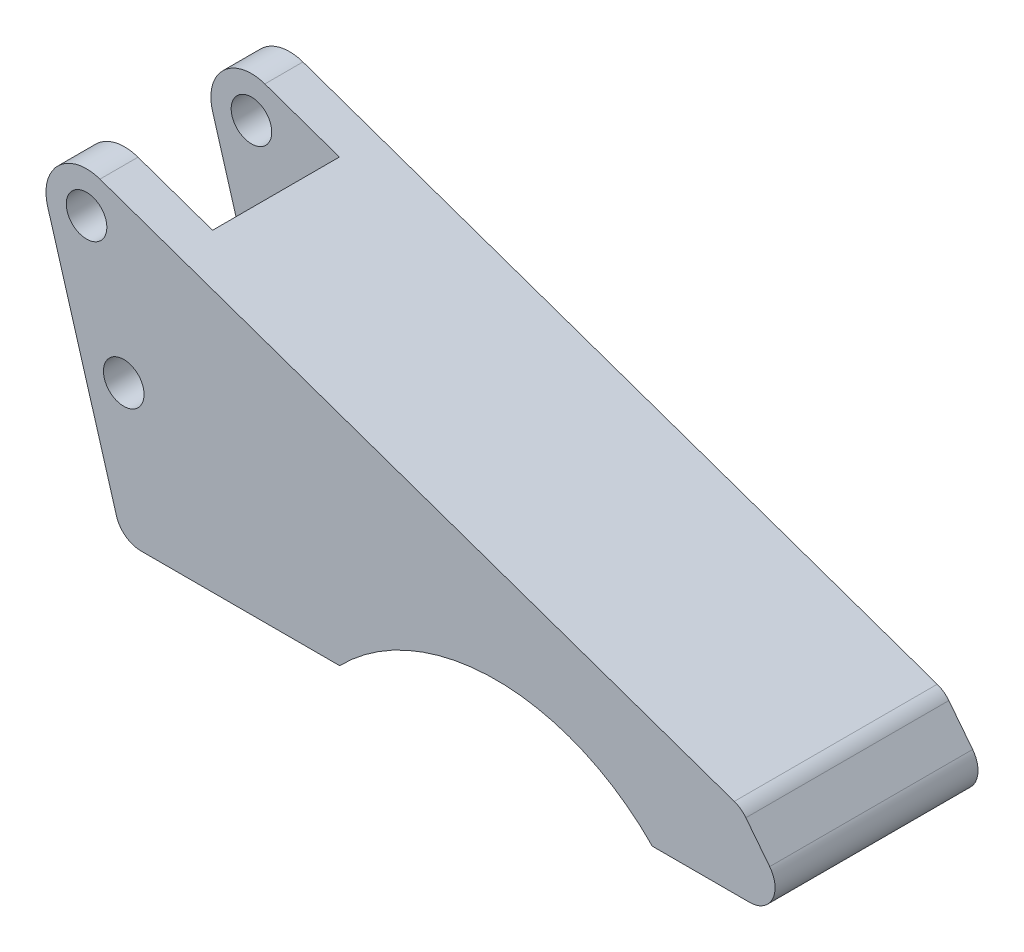
ISO-10303-21;
HEADER;
FILE_DESCRIPTION(('STEP AP214'),'2;1');
FILE_NAME('part.step','',(''),(''),'','','');
FILE_SCHEMA(('AUTOMOTIVE_DESIGN { 1 0 10303 214 1 1 1 1 }'));
ENDSEC;
DATA;
#1=APPLICATION_CONTEXT('core data for automotive mechanical design processes');
#2=APPLICATION_PROTOCOL_DEFINITION('international standard','automotive_design',2000,#1);
#3=PRODUCT_CONTEXT('',#1,'mechanical');
#4=PRODUCT('Part','Part','',(#3));
#5=PRODUCT_RELATED_PRODUCT_CATEGORY('part','',(#4));
#6=PRODUCT_DEFINITION_FORMATION('','',#4);
#7=PRODUCT_DEFINITION_CONTEXT('part definition',#1,'design');
#8=PRODUCT_DEFINITION('design','',#6,#7);
#9=PRODUCT_DEFINITION_SHAPE('','',#8);
#10=(LENGTH_UNIT() NAMED_UNIT(*) SI_UNIT(.MILLI.,.METRE.));
#11=(NAMED_UNIT(*) PLANE_ANGLE_UNIT() SI_UNIT($,.RADIAN.));
#12=(NAMED_UNIT(*) SI_UNIT($,.STERADIAN.) SOLID_ANGLE_UNIT());
#13=UNCERTAINTY_MEASURE_WITH_UNIT(LENGTH_MEASURE(1.E-05),#10,'distance_accuracy_value','');
#14=(GEOMETRIC_REPRESENTATION_CONTEXT(3) GLOBAL_UNCERTAINTY_ASSIGNED_CONTEXT((#13)) GLOBAL_UNIT_ASSIGNED_CONTEXT((#10,
#11,#12)) REPRESENTATION_CONTEXT('',''));
#15=CARTESIAN_POINT('',(0.,0.,0.));
#16=DIRECTION('',(0.,0.,1.));
#17=DIRECTION('',(1.,0.,0.));
#18=AXIS2_PLACEMENT_3D('',#15,#16,#17);
#19=CARTESIAN_POINT('',(-49.8841563985013,51.87,20.));
#20=DIRECTION('',(0.,0.,-1.));
#21=DIRECTION('',(-1.,0.,0.));
#22=AXIS2_PLACEMENT_3D('',#19,#20,#21);
#23=CYLINDRICAL_SURFACE('',#22,7.99999999999999);
#24=CARTESIAN_POINT('',(-49.8841563985013,51.87,12.5));
#25=DIRECTION('',(0.,0.,1.));
#26=DIRECTION('',(1.,0.,0.));
#27=AXIS2_PLACEMENT_3D('',#24,#25,#26);
#28=CIRCLE('',#27,7.99999999999999);
#29=CARTESIAN_POINT('',(-47.2441563985013,59.4218474560865,12.5));
#30=VERTEX_POINT('',#29);
#31=CARTESIAN_POINT('',(-57.5576448104909,49.6077940873871,12.5));
#32=VERTEX_POINT('',#31);
#33=EDGE_CURVE('E230',#30,#32,#28,.T.);
#34=ORIENTED_EDGE('',*,*,#33,.T.);
#35=DIRECTION('',(0.,0.,-1.));
#36=VECTOR('',#35,1.);
#37=CARTESIAN_POINT('',(-57.5576448104909,49.6077940873871,20.));
#38=LINE('',#37,#36);
#39=CARTESIAN_POINT('',(-57.5576448104909,49.6077940873871,20.));
#40=VERTEX_POINT('',#39);
#41=EDGE_CURVE('E192',#40,#32,#38,.T.);
#42=ORIENTED_EDGE('',*,*,#41,.F.);
#43=CARTESIAN_POINT('',(-49.8841563985013,51.87,20.));
#44=DIRECTION('',(0.,0.,1.));
#45=DIRECTION('',(1.,0.,0.));
#46=AXIS2_PLACEMENT_3D('',#43,#44,#45);
#47=CIRCLE('',#46,7.99999999999999);
#48=CARTESIAN_POINT('',(-47.2441563985013,59.4218474560865,20.));
#49=VERTEX_POINT('',#48);
#50=EDGE_CURVE('E143',#49,#40,#47,.T.);
#51=ORIENTED_EDGE('',*,*,#50,.F.);
#52=DIRECTION('',(0.,0.,-1.));
#53=VECTOR('',#52,1.);
#54=CARTESIAN_POINT('',(-47.2441563985013,59.4218474560865,20.));
#55=LINE('',#54,#53);
#56=EDGE_CURVE('E196',#49,#30,#55,.T.);
#57=ORIENTED_EDGE('',*,*,#56,.T.);
#58=EDGE_LOOP('',(#34,#42,#51,#57));
#59=FACE_BOUND('',#58,.T.);
#60=ADVANCED_FACE('F41',(#59),#23,.T.);
#61=CARTESIAN_POINT('',(-43.9900866559948,3.5861213046169,20.));
#62=DIRECTION('',(0.959186051498703,0.282775739076619,0.));
#63=DIRECTION('',(-0.282775739076619,0.959186051498703,0.));
#64=AXIS2_PLACEMENT_3D('',#61,#62,#63);
#65=PLANE('',#64);
#66=DIRECTION('',(0.,0.,-1.));
#67=VECTOR('',#66,1.);
#68=CARTESIAN_POINT('',(-43.9900866559948,3.5861213046169,20.));
#69=LINE('',#68,#67);
#70=CARTESIAN_POINT('',(-43.9900866559948,3.5861213046169,-12.5));
#71=VERTEX_POINT('',#70);
#72=CARTESIAN_POINT('',(-43.9900866559948,3.5861213046169,-20.));
#73=VERTEX_POINT('',#72);
#74=EDGE_CURVE('E156',#71,#73,#69,.T.);
#75=ORIENTED_EDGE('',*,*,#74,.F.);
#76=DIRECTION('',(-0.282775739076619,0.959186051498703,0.));
#77=VECTOR('',#76,1.);
#78=CARTESIAN_POINT('',(-43.9900866559948,3.5861213046169,-12.5));
#79=LINE('',#78,#77);
#80=CARTESIAN_POINT('',(-57.5576448104909,49.6077940873871,-12.5));
#81=VERTEX_POINT('',#80);
#82=EDGE_CURVE('E245',#71,#81,#79,.T.);
#83=ORIENTED_EDGE('',*,*,#82,.T.);
#84=CARTESIAN_POINT('',(-57.5576448104909,49.6077940873871,-20.));
#85=VERTEX_POINT('',#84);
#86=EDGE_CURVE('E154',#81,#85,#38,.T.);
#87=ORIENTED_EDGE('',*,*,#86,.T.);
#88=DIRECTION('',(0.282775739076619,-0.959186051498703,0.));
#89=VECTOR('',#88,1.);
#90=CARTESIAN_POINT('',(-43.9900866559948,3.5861213046169,-20.));
#91=LINE('',#90,#89);
#92=EDGE_CURVE('E184',#85,#73,#91,.T.);
#93=ORIENTED_EDGE('',*,*,#92,.T.);
#94=EDGE_LOOP('',(#75,#83,#87,#93));
#95=FACE_BOUND('',#94,.T.);
#96=ADVANCED_FACE('F321',(#95),#65,.F.);
#97=CARTESIAN_POINT('',(-39.1941563985013,5.,20.));
#98=DIRECTION('',(0.,0.,-1.));
#99=DIRECTION('',(-1.,0.,0.));
#100=AXIS2_PLACEMENT_3D('',#97,#98,#99);
#101=CYLINDRICAL_SURFACE('',#100,5.);
#102=DIRECTION('',(0.,0.,-1.));
#103=VECTOR('',#102,1.);
#104=CARTESIAN_POINT('',(-39.1941563985013,0.,20.));
#105=LINE('',#104,#103);
#106=CARTESIAN_POINT('',(-39.1941563985013,0.,-12.5));
#107=VERTEX_POINT('',#106);
#108=CARTESIAN_POINT('',(-39.1941563985013,0.,-20.));
#109=VERTEX_POINT('',#108);
#110=EDGE_CURVE('E195',#107,#109,#105,.T.);
#111=ORIENTED_EDGE('',*,*,#110,.F.);
#112=CARTESIAN_POINT('',(-39.1941563985013,5.,-12.5));
#113=DIRECTION('',(0.,0.,-1.));
#114=DIRECTION('',(-1.,0.,0.));
#115=AXIS2_PLACEMENT_3D('',#112,#113,#114);
#116=CIRCLE('',#115,5.);
#117=EDGE_CURVE('E238',#107,#71,#116,.T.);
#118=ORIENTED_EDGE('',*,*,#117,.T.);
#119=ORIENTED_EDGE('',*,*,#74,.T.);
#120=CARTESIAN_POINT('',(-39.1941563985013,5.,-20.));
#121=DIRECTION('',(0.,0.,1.));
#122=DIRECTION('',(-1.,0.,0.));
#123=AXIS2_PLACEMENT_3D('',#120,#121,#122);
#124=CIRCLE('',#123,5.);
#125=EDGE_CURVE('E186',#73,#109,#124,.T.);
#126=ORIENTED_EDGE('',*,*,#125,.T.);
#127=EDGE_LOOP('',(#111,#118,#119,#126));
#128=FACE_BOUND('',#127,.T.);
#129=ADVANCED_FACE('F322',(#128),#101,.T.);
#130=CARTESIAN_POINT('',(-49.8841563985013,51.87,20.));
#131=DIRECTION('',(0.,0.,-1.));
#132=DIRECTION('',(-1.,0.,0.));
#133=AXIS2_PLACEMENT_3D('',#130,#131,#132);
#134=CYLINDRICAL_SURFACE('',#133,3.99999999999999);
#135=CARTESIAN_POINT('',(-49.8841563985013,51.87,-12.5));
#136=DIRECTION('',(0.,0.,-1.));
#137=DIRECTION('',(-1.,0.,0.));
#138=AXIS2_PLACEMENT_3D('',#135,#136,#137);
#139=CIRCLE('',#138,3.99999999999999);
#140=CARTESIAN_POINT('',(-53.8841563985013,51.87,-12.5));
#141=VERTEX_POINT('',#140);
#142=EDGE_CURVE('E219',#141,#141,#139,.T.);
#143=ORIENTED_EDGE('',*,*,#142,.F.);
#144=EDGE_LOOP('',(#143));
#145=FACE_BOUND('',#144,.T.);
#146=CARTESIAN_POINT('',(-49.8841563985013,51.87,-20.));
#147=DIRECTION('',(0.,0.,1.));
#148=DIRECTION('',(1.,0.,0.));
#149=AXIS2_PLACEMENT_3D('',#146,#147,#148);
#150=CIRCLE('',#149,3.99999999999999);
#151=CARTESIAN_POINT('',(-45.8841563985013,51.87,-20.));
#152=VERTEX_POINT('',#151);
#153=EDGE_CURVE('E256',#152,#152,#150,.T.);
#154=ORIENTED_EDGE('',*,*,#153,.F.);
#155=EDGE_LOOP('',(#154));
#156=FACE_BOUND('',#155,.T.);
#157=ADVANCED_FACE('F388',(#145,#156),#134,.F.);
#158=CARTESIAN_POINT('',(-42.5541563985013,27.,20.));
#159=DIRECTION('',(0.,0.,-1.));
#160=DIRECTION('',(-1.,0.,0.));
#161=AXIS2_PLACEMENT_3D('',#158,#159,#160);
#162=CYLINDRICAL_SURFACE('',#161,4.);
#163=CARTESIAN_POINT('',(-42.5541563985013,27.,-12.5));
#164=DIRECTION('',(0.,0.,-1.));
#165=DIRECTION('',(-1.,0.,0.));
#166=AXIS2_PLACEMENT_3D('',#163,#164,#165);
#167=CIRCLE('',#166,4.);
#168=CARTESIAN_POINT('',(-46.5541563985013,27.,-12.5));
#169=VERTEX_POINT('',#168);
#170=EDGE_CURVE('E217',#169,#169,#167,.T.);
#171=ORIENTED_EDGE('',*,*,#170,.F.);
#172=EDGE_LOOP('',(#171));
#173=FACE_BOUND('',#172,.T.);
#174=CARTESIAN_POINT('',(-42.5541563985013,27.,-20.));
#175=DIRECTION('',(0.,0.,1.));
#176=DIRECTION('',(1.,0.,0.));
#177=AXIS2_PLACEMENT_3D('',#174,#175,#176);
#178=CIRCLE('',#177,4.);
#179=CARTESIAN_POINT('',(-38.5541563985013,27.,-20.));
#180=VERTEX_POINT('',#179);
#181=EDGE_CURVE('E255',#180,#180,#178,.T.);
#182=ORIENTED_EDGE('',*,*,#181,.F.);
#183=EDGE_LOOP('',(#182));
#184=FACE_BOUND('',#183,.T.);
#185=ADVANCED_FACE('F384',(#173,#184),#162,.F.);
#186=CARTESIAN_POINT('',(30.8058436014987,-30.,20.));
#187=DIRECTION('',(0.,0.,-1.));
#188=DIRECTION('',(-1.,0.,0.));
#189=AXIS2_PLACEMENT_3D('',#186,#187,#188);
#190=PLANE('',#189);
#191=CARTESIAN_POINT('',(30.8058436014987,-30.,20.));
#192=DIRECTION('',(0.,0.,-1.));
#193=DIRECTION('',(-1.,0.,0.));
#194=AXIS2_PLACEMENT_3D('',#191,#192,#193);
#195=CIRCLE('',#194,43.);
#196=CARTESIAN_POINT('',(0.,0.,20.));
#197=VERTEX_POINT('',#196);
#198=CARTESIAN_POINT('',(61.6116872029974,0.,20.));
#199=VERTEX_POINT('',#198);
#200=EDGE_CURVE('E194',#197,#199,#195,.T.);
#201=ORIENTED_EDGE('',*,*,#200,.T.);
#202=DIRECTION('',(1.,0.,0.));
#203=VECTOR('',#202,1.);
#204=CARTESIAN_POINT('',(61.6116872029974,0.,20.));
#205=LINE('',#204,#203);
#206=CARTESIAN_POINT('',(80.8058436014987,0.,20.));
#207=VERTEX_POINT('',#206);
#208=EDGE_CURVE('E115',#199,#207,#205,.T.);
#209=ORIENTED_EDGE('',*,*,#208,.T.);
#210=CARTESIAN_POINT('',(80.8058436014987,5.,20.));
#211=DIRECTION('',(0.,0.,1.));
#212=DIRECTION('',(1.,0.,0.));
#213=AXIS2_PLACEMENT_3D('',#210,#211,#212);
#214=CIRCLE('',#213,5.);
#215=CARTESIAN_POINT('',(84.7456523822993,8.07862092027041,20.));
#216=VERTEX_POINT('',#215);
#217=EDGE_CURVE('E270',#207,#216,#214,.T.);
#218=ORIENTED_EDGE('',*,*,#217,.T.);
#219=DIRECTION('',(-0.615724184054082,0.787961756160116,0.));
#220=VECTOR('',#219,1.);
#221=CARTESIAN_POINT('',(80.0571696286086,14.0786209202704,20.));
#222=LINE('',#221,#220);
#223=CARTESIAN_POINT('',(80.0571696286086,14.0786209202704,20.));
#224=VERTEX_POINT('',#223);
#225=EDGE_CURVE('E267',#216,#224,#222,.T.);
#226=ORIENTED_EDGE('',*,*,#225,.T.);
#227=CARTESIAN_POINT('',(76.1173608478081,11.,20.));
#228=DIRECTION('',(0.,0.,1.));
#229=DIRECTION('',(-1.,0.,0.));
#230=AXIS2_PLACEMENT_3D('',#227,#228,#229);
#231=CIRCLE('',#230,5.);
#232=CARTESIAN_POINT('',(77.767360847808,15.7199046600541,20.));
#233=VERTEX_POINT('',#232);
#234=EDGE_CURVE('E271',#224,#233,#231,.T.);
#235=ORIENTED_EDGE('',*,*,#234,.T.);
#236=DIRECTION('',(-0.943980932010812,0.329999999999998,0.));
#237=VECTOR('',#236,1.);
#238=CARTESIAN_POINT('',(-47.2441563985013,59.4218474560865,20.));
#239=LINE('',#238,#237);
#240=EDGE_CURVE('E272',#233,#49,#239,.T.);
#241=ORIENTED_EDGE('',*,*,#240,.T.);
#242=ORIENTED_EDGE('',*,*,#50,.T.);
#243=DIRECTION('',(0.282775739076619,-0.959186051498703,0.));
#244=VECTOR('',#243,1.);
#245=CARTESIAN_POINT('',(-43.9900866559948,3.5861213046169,20.));
#246=LINE('',#245,#244);
#247=CARTESIAN_POINT('',(-43.9900866559948,3.5861213046169,20.));
#248=VERTEX_POINT('',#247);
#249=EDGE_CURVE('E135',#40,#248,#246,.T.);
#250=ORIENTED_EDGE('',*,*,#249,.T.);
#251=CARTESIAN_POINT('',(-39.1941563985013,5.,20.));
#252=DIRECTION('',(0.,0.,1.));
#253=DIRECTION('',(-1.,0.,0.));
#254=AXIS2_PLACEMENT_3D('',#251,#252,#253);
#255=CIRCLE('',#254,5.);
#256=CARTESIAN_POINT('',(-39.1941563985013,0.,20.));
#257=VERTEX_POINT('',#256);
#258=EDGE_CURVE('E140',#248,#257,#255,.T.);
#259=ORIENTED_EDGE('',*,*,#258,.T.);
#260=DIRECTION('',(1.,0.,0.));
#261=VECTOR('',#260,1.);
#262=CARTESIAN_POINT('',(-39.1941563985013,0.,20.));
#263=LINE('',#262,#261);
#264=EDGE_CURVE('E62',#257,#197,#263,.T.);
#265=ORIENTED_EDGE('',*,*,#264,.T.);
#266=EDGE_LOOP('',(#201,#209,#218,#226,#235,#241,#242,#250,#259,#265));
#267=FACE_BOUND('',#266,.T.);
#268=CARTESIAN_POINT('',(-49.8841563985013,51.87,20.));
#269=DIRECTION('',(0.,0.,1.));
#270=DIRECTION('',(1.,0.,0.));
#271=AXIS2_PLACEMENT_3D('',#268,#269,#270);
#272=CIRCLE('',#271,3.99999999999999);
#273=CARTESIAN_POINT('',(-45.8841563985013,51.87,20.));
#274=VERTEX_POINT('',#273);
#275=EDGE_CURVE('E168',#274,#274,#272,.T.);
#276=ORIENTED_EDGE('',*,*,#275,.F.);
#277=EDGE_LOOP('',(#276));
#278=FACE_BOUND('',#277,.T.);
#279=CARTESIAN_POINT('',(-42.5541563985013,27.,20.));
#280=DIRECTION('',(0.,0.,1.));
#281=DIRECTION('',(1.,0.,0.));
#282=AXIS2_PLACEMENT_3D('',#279,#280,#281);
#283=CIRCLE('',#282,4.);
#284=CARTESIAN_POINT('',(-38.5541563985013,27.,20.));
#285=VERTEX_POINT('',#284);
#286=EDGE_CURVE('E254',#285,#285,#283,.T.);
#287=ORIENTED_EDGE('',*,*,#286,.F.);
#288=EDGE_LOOP('',(#287));
#289=FACE_BOUND('',#288,.T.);
#290=ADVANCED_FACE('F132',(#267,#278,#289),#190,.F.);
#291=CARTESIAN_POINT('',(30.8058436014987,-30.,-20.));
#292=DIRECTION('',(0.,0.,-1.));
#293=DIRECTION('',(-1.,0.,0.));
#294=AXIS2_PLACEMENT_3D('',#291,#292,#293);
#295=PLANE('',#294);
#296=ORIENTED_EDGE('',*,*,#153,.T.);
#297=EDGE_LOOP('',(#296));
#298=FACE_BOUND('',#297,.T.);
#299=CARTESIAN_POINT('',(30.8058436014987,-30.,-20.));
#300=DIRECTION('',(0.,0.,-1.));
#301=DIRECTION('',(-1.,0.,0.));
#302=AXIS2_PLACEMENT_3D('',#299,#300,#301);
#303=CIRCLE('',#302,43.);
#304=CARTESIAN_POINT('',(0.,0.,-20.));
#305=VERTEX_POINT('',#304);
#306=CARTESIAN_POINT('',(61.6116872029974,0.,-20.));
#307=VERTEX_POINT('',#306);
#308=EDGE_CURVE('E167',#305,#307,#303,.T.);
#309=ORIENTED_EDGE('',*,*,#308,.F.);
#310=DIRECTION('',(1.,0.,0.));
#311=VECTOR('',#310,1.);
#312=CARTESIAN_POINT('',(-39.1941563985013,0.,-20.));
#313=LINE('',#312,#311);
#314=EDGE_CURVE('E103',#109,#305,#313,.T.);
#315=ORIENTED_EDGE('',*,*,#314,.F.);
#316=ORIENTED_EDGE('',*,*,#125,.F.);
#317=ORIENTED_EDGE('',*,*,#92,.F.);
#318=CARTESIAN_POINT('',(-49.8841563985013,51.87,-20.));
#319=DIRECTION('',(0.,0.,1.));
#320=DIRECTION('',(1.,0.,0.));
#321=AXIS2_PLACEMENT_3D('',#318,#319,#320);
#322=CIRCLE('',#321,7.99999999999999);
#323=CARTESIAN_POINT('',(-47.2441563985013,59.4218474560865,-20.));
#324=VERTEX_POINT('',#323);
#325=EDGE_CURVE('E182',#324,#85,#322,.T.);
#326=ORIENTED_EDGE('',*,*,#325,.F.);
#327=DIRECTION('',(-0.943980932010812,0.329999999999998,0.));
#328=VECTOR('',#327,1.);
#329=CARTESIAN_POINT('',(-47.2441563985013,59.4218474560865,-20.));
#330=LINE('',#329,#328);
#331=CARTESIAN_POINT('',(77.767360847808,15.7199046600541,-20.));
#332=VERTEX_POINT('',#331);
#333=EDGE_CURVE('E180',#332,#324,#330,.T.);
#334=ORIENTED_EDGE('',*,*,#333,.F.);
#335=CARTESIAN_POINT('',(76.1173608478081,11.,-20.));
#336=DIRECTION('',(0.,0.,1.));
#337=DIRECTION('',(-1.,0.,0.));
#338=AXIS2_PLACEMENT_3D('',#335,#336,#337);
#339=CIRCLE('',#338,5.);
#340=CARTESIAN_POINT('',(80.0571696286086,14.0786209202704,-20.));
#341=VERTEX_POINT('',#340);
#342=EDGE_CURVE('E179',#341,#332,#339,.T.);
#343=ORIENTED_EDGE('',*,*,#342,.F.);
#344=DIRECTION('',(-0.615724184054082,0.787961756160116,0.));
#345=VECTOR('',#344,1.);
#346=CARTESIAN_POINT('',(80.0571696286086,14.0786209202704,-20.));
#347=LINE('',#346,#345);
#348=CARTESIAN_POINT('',(84.7456523822993,8.07862092027041,-20.));
#349=VERTEX_POINT('',#348);
#350=EDGE_CURVE('E173',#349,#341,#347,.T.);
#351=ORIENTED_EDGE('',*,*,#350,.F.);
#352=CARTESIAN_POINT('',(80.8058436014987,5.,-20.));
#353=DIRECTION('',(0.,0.,1.));
#354=DIRECTION('',(1.,0.,0.));
#355=AXIS2_PLACEMENT_3D('',#352,#353,#354);
#356=CIRCLE('',#355,5.);
#357=CARTESIAN_POINT('',(80.8058436014987,0.,-20.));
#358=VERTEX_POINT('',#357);
#359=EDGE_CURVE('E171',#358,#349,#356,.T.);
#360=ORIENTED_EDGE('',*,*,#359,.F.);
#361=DIRECTION('',(1.,0.,0.));
#362=VECTOR('',#361,1.);
#363=CARTESIAN_POINT('',(61.6116872029974,0.,-20.));
#364=LINE('',#363,#362);
#365=EDGE_CURVE('E166',#307,#358,#364,.T.);
#366=ORIENTED_EDGE('',*,*,#365,.F.);
#367=EDGE_LOOP('',(#309,#315,#316,#317,#326,#334,#343,#351,#360,#366));
#368=FACE_BOUND('',#367,.T.);
#369=ORIENTED_EDGE('',*,*,#181,.T.);
#370=EDGE_LOOP('',(#369));
#371=FACE_BOUND('',#370,.T.);
#372=ADVANCED_FACE('F316',(#298,#368,#371),#295,.T.);
#373=CARTESIAN_POINT('',(30.8058436014987,-30.,20.));
#374=DIRECTION('',(0.,0.,-1.));
#375=DIRECTION('',(-1.,0.,0.));
#376=AXIS2_PLACEMENT_3D('',#373,#374,#375);
#377=CYLINDRICAL_SURFACE('',#376,43.);
#378=ORIENTED_EDGE('',*,*,#308,.T.);
#379=DIRECTION('',(0.,0.,-1.));
#380=VECTOR('',#379,1.);
#381=CARTESIAN_POINT('',(61.6116872029974,0.,20.));
#382=LINE('',#381,#380);
#383=EDGE_CURVE('E47',#199,#307,#382,.T.);
#384=ORIENTED_EDGE('',*,*,#383,.F.);
#385=ORIENTED_EDGE('',*,*,#200,.F.);
#386=DIRECTION('',(0.,0.,-1.));
#387=VECTOR('',#386,1.);
#388=CARTESIAN_POINT('',(0.,0.,20.));
#389=LINE('',#388,#387);
#390=EDGE_CURVE('E165',#197,#305,#389,.T.);
#391=ORIENTED_EDGE('',*,*,#390,.T.);
#392=EDGE_LOOP('',(#378,#384,#385,#391));
#393=FACE_BOUND('',#392,.T.);
#394=ADVANCED_FACE('F43',(#393),#377,.F.);
#395=CARTESIAN_POINT('',(61.6116872029974,0.,20.));
#396=DIRECTION('',(0.,1.,0.));
#397=DIRECTION('',(0.,0.,1.));
#398=AXIS2_PLACEMENT_3D('',#395,#396,#397);
#399=PLANE('',#398);
#400=ORIENTED_EDGE('',*,*,#365,.T.);
#401=DIRECTION('',(0.,0.,-1.));
#402=VECTOR('',#401,1.);
#403=CARTESIAN_POINT('',(80.8058436014987,0.,20.));
#404=LINE('',#403,#402);
#405=EDGE_CURVE('E209',#207,#358,#404,.T.);
#406=ORIENTED_EDGE('',*,*,#405,.F.);
#407=ORIENTED_EDGE('',*,*,#208,.F.);
#408=ORIENTED_EDGE('',*,*,#383,.T.);
#409=EDGE_LOOP('',(#400,#406,#407,#408));
#410=FACE_BOUND('',#409,.T.);
#411=ADVANCED_FACE('F345',(#410),#399,.F.);
#412=CARTESIAN_POINT('',(80.8058436014987,5.,20.));
#413=DIRECTION('',(0.,0.,-1.));
#414=DIRECTION('',(-1.,0.,0.));
#415=AXIS2_PLACEMENT_3D('',#412,#413,#414);
#416=CYLINDRICAL_SURFACE('',#415,5.);
#417=ORIENTED_EDGE('',*,*,#359,.T.);
#418=DIRECTION('',(0.,0.,-1.));
#419=VECTOR('',#418,1.);
#420=CARTESIAN_POINT('',(84.7456523822993,8.07862092027041,20.));
#421=LINE('',#420,#419);
#422=EDGE_CURVE('E210',#216,#349,#421,.T.);
#423=ORIENTED_EDGE('',*,*,#422,.F.);
#424=ORIENTED_EDGE('',*,*,#217,.F.);
#425=ORIENTED_EDGE('',*,*,#405,.T.);
#426=EDGE_LOOP('',(#417,#423,#424,#425));
#427=FACE_BOUND('',#426,.T.);
#428=ADVANCED_FACE('F347',(#427),#416,.T.);
#429=CARTESIAN_POINT('',(80.0571696286086,14.0786209202704,20.));
#430=DIRECTION('',(-0.787961756160116,-0.615724184054082,0.));
#431=DIRECTION('',(0.615724184054082,-0.787961756160116,0.));
#432=AXIS2_PLACEMENT_3D('',#429,#430,#431);
#433=PLANE('',#432);
#434=ORIENTED_EDGE('',*,*,#350,.T.);
#435=DIRECTION('',(0.,0.,-1.));
#436=VECTOR('',#435,1.);
#437=CARTESIAN_POINT('',(80.0571696286086,14.0786209202704,20.));
#438=LINE('',#437,#436);
#439=EDGE_CURVE('E204',#224,#341,#438,.T.);
#440=ORIENTED_EDGE('',*,*,#439,.F.);
#441=ORIENTED_EDGE('',*,*,#225,.F.);
#442=ORIENTED_EDGE('',*,*,#422,.T.);
#443=EDGE_LOOP('',(#434,#440,#441,#442));
#444=FACE_BOUND('',#443,.T.);
#445=ADVANCED_FACE('F354',(#444),#433,.F.);
#446=CARTESIAN_POINT('',(76.1173608478081,11.,20.));
#447=DIRECTION('',(0.,0.,-1.));
#448=DIRECTION('',(-1.,0.,0.));
#449=AXIS2_PLACEMENT_3D('',#446,#447,#448);
#450=CYLINDRICAL_SURFACE('',#449,5.);
#451=ORIENTED_EDGE('',*,*,#342,.T.);
#452=DIRECTION('',(0.,0.,-1.));
#453=VECTOR('',#452,1.);
#454=CARTESIAN_POINT('',(77.767360847808,15.7199046600541,20.));
#455=LINE('',#454,#453);
#456=EDGE_CURVE('E203',#233,#332,#455,.T.);
#457=ORIENTED_EDGE('',*,*,#456,.F.);
#458=ORIENTED_EDGE('',*,*,#234,.F.);
#459=ORIENTED_EDGE('',*,*,#439,.T.);
#460=EDGE_LOOP('',(#451,#457,#458,#459));
#461=FACE_BOUND('',#460,.T.);
#462=ADVANCED_FACE('F355',(#461),#450,.T.);
#463=CARTESIAN_POINT('',(-47.2441563985013,59.4218474560865,20.));
#464=DIRECTION('',(-0.329999999999998,-0.943980932010812,0.));
#465=DIRECTION('',(0.943980932010812,-0.329999999999998,0.));
#466=AXIS2_PLACEMENT_3D('',#463,#464,#465);
#467=PLANE('',#466);
#468=CARTESIAN_POINT('',(-47.2441563985013,59.4218474560865,-12.5));
#469=VERTEX_POINT('',#468);
#470=EDGE_CURVE('E197',#469,#324,#55,.T.);
#471=ORIENTED_EDGE('',*,*,#470,.F.);
#472=DIRECTION('',(0.943980932010812,-0.329999999999998,0.));
#473=VECTOR('',#472,1.);
#474=CARTESIAN_POINT('',(-47.2441563985013,59.4218474560865,-12.5));
#475=LINE('',#474,#473);
#476=CARTESIAN_POINT('',(-32.5576448104909,54.287687792798,-12.5));
#477=VERTEX_POINT('',#476);
#478=EDGE_CURVE('E248',#469,#477,#475,.T.);
#479=ORIENTED_EDGE('',*,*,#478,.T.);
#480=DIRECTION('',(0.,0.,1.));
#481=VECTOR('',#480,1.);
#482=CARTESIAN_POINT('',(-32.5576448104909,54.287687792798,20.));
#483=LINE('',#482,#481);
#484=CARTESIAN_POINT('',(-32.5576448104909,54.287687792798,12.5));
#485=VERTEX_POINT('',#484);
#486=EDGE_CURVE('E252',#477,#485,#483,.T.);
#487=ORIENTED_EDGE('',*,*,#486,.T.);
#488=DIRECTION('',(-0.943980932010812,0.329999999999998,0.));
#489=VECTOR('',#488,1.);
#490=CARTESIAN_POINT('',(-47.2441563985013,59.4218474560865,12.5));
#491=LINE('',#490,#489);
#492=EDGE_CURVE('E222',#485,#30,#491,.T.);
#493=ORIENTED_EDGE('',*,*,#492,.T.);
#494=ORIENTED_EDGE('',*,*,#56,.F.);
#495=ORIENTED_EDGE('',*,*,#240,.F.);
#496=ORIENTED_EDGE('',*,*,#456,.T.);
#497=ORIENTED_EDGE('',*,*,#333,.T.);
#498=EDGE_LOOP('',(#471,#479,#487,#493,#494,#495,#496,#497));
#499=FACE_BOUND('',#498,.T.);
#500=ADVANCED_FACE('F279',(#499),#467,.F.);
#501=ORIENTED_EDGE('',*,*,#86,.F.);
#502=CARTESIAN_POINT('',(-49.8841563985013,51.87,-12.5));
#503=DIRECTION('',(0.,0.,-1.));
#504=DIRECTION('',(-1.,0.,0.));
#505=AXIS2_PLACEMENT_3D('',#502,#503,#504);
#506=CIRCLE('',#505,7.99999999999999);
#507=EDGE_CURVE('E249',#81,#469,#506,.T.);
#508=ORIENTED_EDGE('',*,*,#507,.T.);
#509=ORIENTED_EDGE('',*,*,#470,.T.);
#510=ORIENTED_EDGE('',*,*,#325,.T.);
#511=EDGE_LOOP('',(#501,#508,#509,#510));
#512=FACE_BOUND('',#511,.T.);
#513=ADVANCED_FACE('F310',(#512),#23,.T.);
#514=ORIENTED_EDGE('',*,*,#41,.T.);
#515=DIRECTION('',(0.282775739076619,-0.959186051498703,0.));
#516=VECTOR('',#515,1.);
#517=CARTESIAN_POINT('',(-43.9900866559948,3.5861213046169,12.5));
#518=LINE('',#517,#516);
#519=CARTESIAN_POINT('',(-43.9900866559948,3.5861213046169,12.5));
#520=VERTEX_POINT('',#519);
#521=EDGE_CURVE('E155',#32,#520,#518,.T.);
#522=ORIENTED_EDGE('',*,*,#521,.T.);
#523=EDGE_CURVE('E146',#248,#520,#69,.T.);
#524=ORIENTED_EDGE('',*,*,#523,.F.);
#525=ORIENTED_EDGE('',*,*,#249,.F.);
#526=EDGE_LOOP('',(#514,#522,#524,#525));
#527=FACE_BOUND('',#526,.T.);
#528=ADVANCED_FACE('F149',(#527),#65,.F.);
#529=ORIENTED_EDGE('',*,*,#523,.T.);
#530=CARTESIAN_POINT('',(-39.1941563985013,5.,12.5));
#531=DIRECTION('',(0.,0.,1.));
#532=DIRECTION('',(1.,0.,0.));
#533=AXIS2_PLACEMENT_3D('',#530,#531,#532);
#534=CIRCLE('',#533,5.);
#535=CARTESIAN_POINT('',(-39.1941563985013,0.,12.5));
#536=VERTEX_POINT('',#535);
#537=EDGE_CURVE('E339',#520,#536,#534,.T.);
#538=ORIENTED_EDGE('',*,*,#537,.T.);
#539=EDGE_CURVE('E159',#257,#536,#105,.T.);
#540=ORIENTED_EDGE('',*,*,#539,.F.);
#541=ORIENTED_EDGE('',*,*,#258,.F.);
#542=EDGE_LOOP('',(#529,#538,#540,#541));
#543=FACE_BOUND('',#542,.T.);
#544=ADVANCED_FACE('F158',(#543),#101,.T.);
#545=CARTESIAN_POINT('',(-39.1941563985013,0.,20.));
#546=DIRECTION('',(0.,1.,0.));
#547=DIRECTION('',(0.,0.,1.));
#548=AXIS2_PLACEMENT_3D('',#545,#546,#547);
#549=PLANE('',#548);
#550=DIRECTION('',(0.,0.,-1.));
#551=VECTOR('',#550,1.);
#552=CARTESIAN_POINT('',(-32.5576448104909,0.,20.));
#553=LINE('',#552,#551);
#554=CARTESIAN_POINT('',(-32.5576448104909,0.,12.5));
#555=VERTEX_POINT('',#554);
#556=CARTESIAN_POINT('',(-32.5576448104909,0.,-12.5));
#557=VERTEX_POINT('',#556);
#558=EDGE_CURVE('E11',#555,#557,#553,.T.);
#559=ORIENTED_EDGE('',*,*,#558,.T.);
#560=DIRECTION('',(-1.,0.,0.));
#561=VECTOR('',#560,1.);
#562=CARTESIAN_POINT('',(-39.1941563985013,0.,-12.5));
#563=LINE('',#562,#561);
#564=EDGE_CURVE('E223',#557,#107,#563,.T.);
#565=ORIENTED_EDGE('',*,*,#564,.T.);
#566=ORIENTED_EDGE('',*,*,#110,.T.);
#567=ORIENTED_EDGE('',*,*,#314,.T.);
#568=ORIENTED_EDGE('',*,*,#390,.F.);
#569=ORIENTED_EDGE('',*,*,#264,.F.);
#570=ORIENTED_EDGE('',*,*,#539,.T.);
#571=DIRECTION('',(1.,0.,0.));
#572=VECTOR('',#571,1.);
#573=CARTESIAN_POINT('',(-39.1941563985013,0.,12.5));
#574=LINE('',#573,#572);
#575=EDGE_CURVE('E331',#536,#555,#574,.T.);
#576=ORIENTED_EDGE('',*,*,#575,.T.);
#577=EDGE_LOOP('',(#559,#565,#566,#567,#568,#569,#570,#576));
#578=FACE_BOUND('',#577,.T.);
#579=ADVANCED_FACE('F324',(#578),#549,.F.);
#580=CARTESIAN_POINT('',(-49.8841563985013,51.87,12.5));
#581=DIRECTION('',(0.,0.,1.));
#582=DIRECTION('',(1.,0.,0.));
#583=AXIS2_PLACEMENT_3D('',#580,#581,#582);
#584=CIRCLE('',#583,3.99999999999999);
#585=CARTESIAN_POINT('',(-45.8841563985013,51.87,12.5));
#586=VERTEX_POINT('',#585);
#587=EDGE_CURVE('E216',#586,#586,#584,.T.);
#588=ORIENTED_EDGE('',*,*,#587,.F.);
#589=EDGE_LOOP('',(#588));
#590=FACE_BOUND('',#589,.T.);
#591=ORIENTED_EDGE('',*,*,#275,.T.);
#592=EDGE_LOOP('',(#591));
#593=FACE_BOUND('',#592,.T.);
#594=ADVANCED_FACE('F377',(#590,#593),#134,.F.);
#595=CARTESIAN_POINT('',(-42.5541563985013,27.,12.5));
#596=DIRECTION('',(0.,0.,1.));
#597=DIRECTION('',(1.,0.,0.));
#598=AXIS2_PLACEMENT_3D('',#595,#596,#597);
#599=CIRCLE('',#598,4.);
#600=CARTESIAN_POINT('',(-38.5541563985013,27.,12.5));
#601=VERTEX_POINT('',#600);
#602=EDGE_CURVE('E212',#601,#601,#599,.T.);
#603=ORIENTED_EDGE('',*,*,#602,.F.);
#604=EDGE_LOOP('',(#603));
#605=FACE_BOUND('',#604,.T.);
#606=ORIENTED_EDGE('',*,*,#286,.T.);
#607=EDGE_LOOP('',(#606));
#608=FACE_BOUND('',#607,.T.);
#609=ADVANCED_FACE('F389',(#605,#608),#162,.F.);
#610=CARTESIAN_POINT('',(-32.5576448104909,59.87,-12.5));
#611=DIRECTION('',(1.,0.,0.));
#612=DIRECTION('',(0.,0.,-1.));
#613=AXIS2_PLACEMENT_3D('',#610,#611,#612);
#614=PLANE('',#613);
#615=DIRECTION('',(0.,-1.,0.));
#616=VECTOR('',#615,1.);
#617=CARTESIAN_POINT('',(-32.5576448104909,59.87,-12.5));
#618=LINE('',#617,#616);
#619=EDGE_CURVE('E220',#477,#557,#618,.T.);
#620=ORIENTED_EDGE('',*,*,#619,.T.);
#621=ORIENTED_EDGE('',*,*,#558,.F.);
#622=DIRECTION('',(0.,-1.,0.));
#623=VECTOR('',#622,1.);
#624=CARTESIAN_POINT('',(-32.5576448104909,59.87,12.5));
#625=LINE('',#624,#623);
#626=EDGE_CURVE('E57',#485,#555,#625,.T.);
#627=ORIENTED_EDGE('',*,*,#626,.F.);
#628=ORIENTED_EDGE('',*,*,#486,.F.);
#629=EDGE_LOOP('',(#620,#621,#627,#628));
#630=FACE_BOUND('',#629,.T.);
#631=ADVANCED_FACE('F327',(#630),#614,.F.);
#632=CARTESIAN_POINT('',(-82.5576448104909,59.87,-12.5));
#633=DIRECTION('',(0.,0.,-1.));
#634=DIRECTION('',(-1.,0.,0.));
#635=AXIS2_PLACEMENT_3D('',#632,#633,#634);
#636=PLANE('',#635);
#637=ORIENTED_EDGE('',*,*,#142,.T.);
#638=EDGE_LOOP('',(#637));
#639=FACE_BOUND('',#638,.T.);
#640=ORIENTED_EDGE('',*,*,#170,.T.);
#641=EDGE_LOOP('',(#640));
#642=FACE_BOUND('',#641,.T.);
#643=ORIENTED_EDGE('',*,*,#507,.F.);
#644=ORIENTED_EDGE('',*,*,#82,.F.);
#645=ORIENTED_EDGE('',*,*,#117,.F.);
#646=ORIENTED_EDGE('',*,*,#564,.F.);
#647=ORIENTED_EDGE('',*,*,#619,.F.);
#648=ORIENTED_EDGE('',*,*,#478,.F.);
#649=EDGE_LOOP('',(#643,#644,#645,#646,#647,#648));
#650=FACE_BOUND('',#649,.T.);
#651=ADVANCED_FACE('F302',(#639,#642,#650),#636,.F.);
#652=CARTESIAN_POINT('',(-82.5576448104909,59.87,12.5));
#653=DIRECTION('',(0.,0.,1.));
#654=DIRECTION('',(1.,0.,0.));
#655=AXIS2_PLACEMENT_3D('',#652,#653,#654);
#656=PLANE('',#655);
#657=ORIENTED_EDGE('',*,*,#587,.T.);
#658=EDGE_LOOP('',(#657));
#659=FACE_BOUND('',#658,.T.);
#660=ORIENTED_EDGE('',*,*,#602,.T.);
#661=EDGE_LOOP('',(#660));
#662=FACE_BOUND('',#661,.T.);
#663=ORIENTED_EDGE('',*,*,#626,.T.);
#664=ORIENTED_EDGE('',*,*,#575,.F.);
#665=ORIENTED_EDGE('',*,*,#537,.F.);
#666=ORIENTED_EDGE('',*,*,#521,.F.);
#667=ORIENTED_EDGE('',*,*,#33,.F.);
#668=ORIENTED_EDGE('',*,*,#492,.F.);
#669=EDGE_LOOP('',(#663,#664,#665,#666,#667,#668));
#670=FACE_BOUND('',#669,.T.);
#671=ADVANCED_FACE('F399',(#659,#662,#670),#656,.F.);
#672=CLOSED_SHELL('',(#60,#96,#129,#157,#185,#290,#372,#394,#411,#428,#445,#462,#500,#513,#528,
#544,#579,#594,#609,#631,#651,#671));
#673=MANIFOLD_SOLID_BREP('B2',#672);
#674=ADVANCED_BREP_SHAPE_REPRESENTATION('',(#18,#673),#14);
#675=SHAPE_DEFINITION_REPRESENTATION(#9,#674);
ENDSEC;
END-ISO-10303-21;
